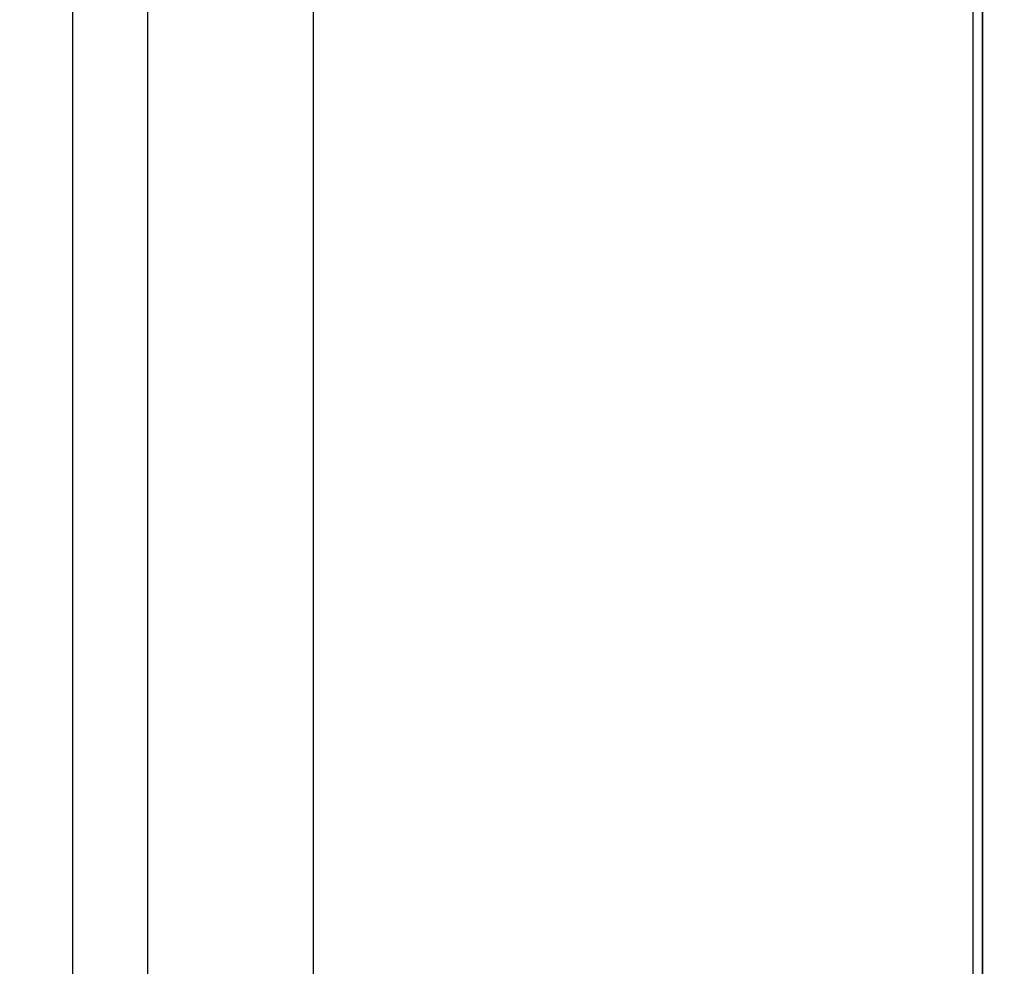
# Model space of a CAD drawing. Units: inches. Extents: x 844 to 2234, y 346 to 1084.
# Tile 24 of 93: x 1136 to 1189, y 680 to 731. Entities that reach past the tile are written whole.
import ezdxf

# ---------------------------------------------------------------- set-up
doc = ezdxf.new("R2010")
doc.units = ezdxf.units.IN
doc.header["$MEASUREMENT"] = 0
doc.layers.add('A-ANNO-DIMS', color=2, linetype='Continuous', lineweight=18)
doc.layers.add('A-WALL', color=7, linetype='Continuous', lineweight=35)
doc.styles.get("Standard").update_dxf_attribs({"font": 'arial.ttf'})
doc.dimstyles.get("Standard").update_dxf_attribs({"dimtxt": 6, "dimasz": 3, "dimexe": 0.18, "dimexo": 0.0625, "dimgap": 0.09, "dimtad": 0, "dimtih": 1, "dimtoh": 1, "dimdec": 1, "dimzin": 0, "dimdsep": 46, "dimlunit": 3, "dimtxsty": 'Standard', "dimblk": 'ARCHTICK', "dimcen": 0.09, "dimadec": 0, "dimazin": 0, "dimtfac": 1, "dimtdec": 1, "dimtofl": 0, "dimtmove": 0, "dimatfit": 3, "dimfxl": 1, "dimtolj": 1, "dimtzin": 0, "dimarcsym": 0})

# ---------------------------------------------------------------- blocks, each defined once
blk = doc.blocks.new('_ArchTick')
at = {"color": 0, "linetype": 'ByBlock', "const_width": 0.15}
blk.add_lwpolyline([(-0.5, -0.5), (0.5, 0.5)], dxfattribs=at)
blk = doc.blocks.new('*D54')
at = {"layer": 'A-ANNO-DIMS', "color": 0, "lineweight": -2, "transparency": 16777216}
for p, q in [((1139.678, 879.311), (1152.117, 879.311)), ((1151.937, 879.311), (1151.937, 758.401)), ((1151.937, 631.184), (1151.937, 752.094)), ((1139.678, 631.184), (1152.117, 631.184))]:
    blk.add_line(p, q, dxfattribs=at)
at = {"layer": 'Defpoints', "color": 0, "transparency": 16777216}
for p in [(1139.616, 879.311), (1139.616, 631.184), (1151.937, 631.184)]:
    blk.add_point(p, dxfattribs=at)
at = {"layer": 'A-ANNO-DIMS', "color": 0, "lineweight": -2, "transparency": 16777216, "xscale": 3, "yscale": 3, "zscale": 3}
for p, rotation in [((1151.937, 879.311), 90), ((1151.937, 631.184), 270)]:
    blk.add_blockref('_ArchTick', p, dxfattribs=dict(at, rotation=rotation))
at = {"layer": 'A-ANNO-DIMS', "color": 0, "transparency": 16777216, "insert": (1151.937, 755.248), "char_height": 6, "attachment_point": 5}
blk.add_mtext('\\A1;20\'-8.1"', dxfattribs=at)
blk = doc.blocks.new('*D143')
at = {"layer": 'A-ANNO-DIMS', "color": 0, "lineweight": -2, "transparency": 16777216}
for p, q in [((1139.116, 430.373), (1139.116, 1074.743)), ((1187.116, 430.373), (1187.116, 1074.743)), ((1139.116, 1074.563), (1154.93, 1074.563)), ((1187.116, 1074.563), (1171.301, 1074.563))]:
    blk.add_line(p, q, dxfattribs=at)
at = {"layer": 'Defpoints', "color": 0, "transparency": 16777216}
for p in [(1187.116, 1074.563), (1139.116, 430.311), (1187.116, 430.311)]:
    blk.add_point(p, dxfattribs=at)
at = {"layer": 'A-ANNO-DIMS', "color": 0, "lineweight": -2, "transparency": 16777216, "xscale": 3, "yscale": 3, "zscale": 3, "rotation": 180}
blk.add_blockref('_ArchTick', (1139.116, 1074.563), dxfattribs=at)
at = {"layer": 'A-ANNO-DIMS', "color": 0, "lineweight": -2, "transparency": 16777216, "xscale": 3, "yscale": 3, "zscale": 3}
blk.add_blockref('_ArchTick', (1187.116, 1074.563), dxfattribs=at)
at = {"layer": 'A-ANNO-DIMS', "color": 0, "transparency": 16777216, "insert": (1163.116, 1074.563), "char_height": 6, "attachment_point": 5}
blk.add_mtext('\\A1;4\'-0"', dxfattribs=at)
blk = doc.blocks.new('*D144')
at = {"layer": 'A-ANNO-DIMS', "color": 0, "lineweight": -2, "transparency": 16777216}
for p, q in [((1096.616, 439.373), (1096.616, 1074.743)), ((1143.116, 492.373), (1143.116, 1074.743)), ((1096.616, 1074.563), (1102.482, 1074.563)), ((1143.116, 1074.563), (1137.25, 1074.563))]:
    blk.add_line(p, q, dxfattribs=at)
at = {"layer": 'Defpoints', "color": 0, "transparency": 16777216}
for p in [(1143.116, 1074.563), (1143.116, 492.311), (1096.616, 439.311)]:
    blk.add_point(p, dxfattribs=at)
at = {"layer": 'A-ANNO-DIMS', "color": 0, "lineweight": -2, "transparency": 16777216, "xscale": 3, "yscale": 3, "zscale": 3, "rotation": 180}
blk.add_blockref('_ArchTick', (1096.616, 1074.563), dxfattribs=at)
at = {"layer": 'A-ANNO-DIMS', "color": 0, "lineweight": -2, "transparency": 16777216, "xscale": 3, "yscale": 3, "zscale": 3}
blk.add_blockref('_ArchTick', (1143.116, 1074.563), dxfattribs=at)
at = {"layer": 'A-ANNO-DIMS', "color": 0, "transparency": 16777216, "insert": (1119.866, 1074.563), "char_height": 6, "attachment_point": 5}
blk.add_mtext('\\A1;3\'-10 1/2"', dxfattribs=at)

msp = doc.modelspace()

# ---------------------------------------------------------------- linework, layer by layer
at = {"layer": 'A-WALL'}
msp.add_line((1187.616, 766.311), (1187.616, 629.311), dxfattribs=at)

# ---------------------------------------------------------------- dimensions: what is measured, and where the dimension line sits
at = {"layer": 'A-ANNO-DIMS'}
for base, p1, p2, picture, middle in [((1143.116, 1074.563), (1096.616, 439.311), (1143.116, 492.311), '*D144', (1119.866, 1074.563)), ((1187.116, 1074.563), (1139.116, 430.311), (1187.116, 430.311), '*D143', (1163.116, 1074.563))]:
    dim = msp.add_linear_dim(base=base, p1=p1, p2=p2, dimstyle='Standard', override={"dimdec": 1, "dimlfac": 1, "dimrnd": 0, "dimzin": 1, "dimdsep": 46, "dimlunit": 4, "dimfrac": 2}, dxfattribs=at)
    dim.commit()
    dim.dimension.update_dxf_attribs({"geometry": picture, "text_midpoint": middle})
dim = msp.add_linear_dim(base=(1151.937, 631.184), p1=(1139.616, 879.311), p2=(1139.616, 631.184), angle=90, dimstyle='Standard', override={"dimclrd": 0, "dimclre": 0, "dimclrt": 0}, dxfattribs=at)
dim.commit()
dim.dimension.update_dxf_attribs({"geometry": '*D54', "text_midpoint": (1151.937, 755.248)})

doc.saveas('drawing.dxf')
